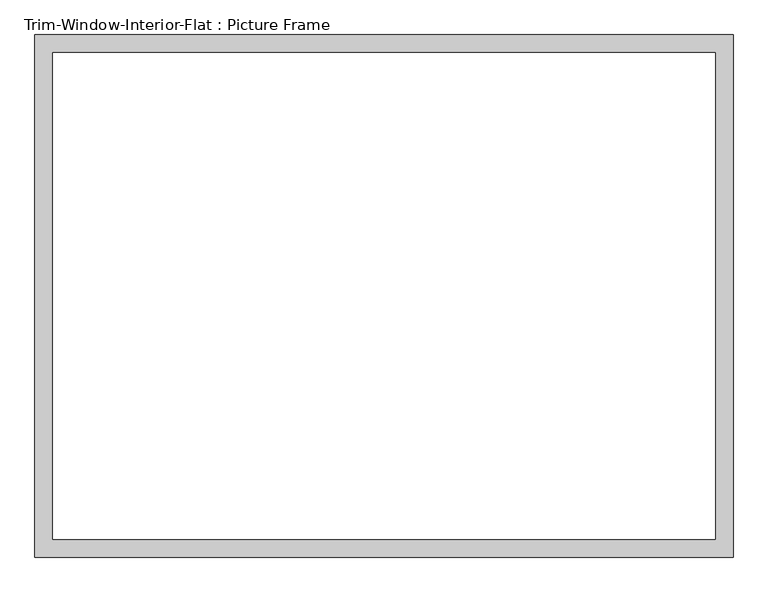
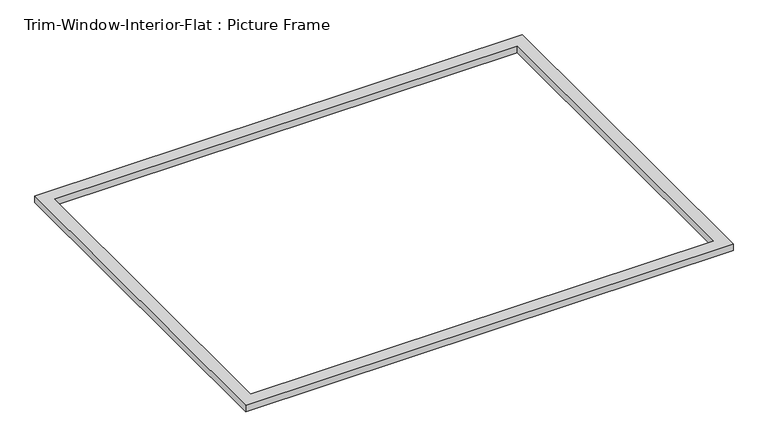
"""IFC4 building model written with IfcOpenShell, lengths in millimetres: proxy geometry, Trim-Window-Interior-Flat : Picture Frame."""

from ifc_helpers import new_model, si_unit, origin, origin_with_axes, place, context, project, spatial, polyline, outline, extrude, source, transform, mapped, element, save


def trim_window_interior_flat_picture_frame_e25f2530(model_context):
    return source(origin(), model_context, "Body", "SweptSolid", [
        extrude(outline(polyline([(1111.25, 44.45), (1111.25, -1619.25), (-1111.25, -1619.25), (-1111.25, 44.45), (1111.25, 44.45)]), holes=[polyline([(1054.1, -12.7), (-1054.1, -12.7), (-1054.1, -1562.1), (1054.1, -1562.1), (1054.1, -12.7)])]), origin_with_axes(), (0.0, 0.0, 1.0), 31.75),
    ])


if __name__ == "__main__":
    model = new_model("IFC4")
    model_context = context("Model", 3, world=origin())
    ifc_project = project(units=[si_unit("LENGTHUNIT", "METRE", prefix="MILLI")], contexts=[model_context])
    site = spatial("IfcSite", under=ifc_project)
    building = spatial("IfcBuilding", under=site)
    placement = place(None, origin())
    trim_window_interior_flat_picture_frame_shape = trim_window_interior_flat_picture_frame_e25f2530(model_context)
    element("IfcBuildingElementProxy", 1, Name="Trim-Window-Interior-Flat : Picture Frame", ObjectType="Trim-Window-Interior-Flat : Picture Frame", at=placement, inside=building, context=model_context, shape_type="MappedRepresentation", body=[
        mapped(trim_window_interior_flat_picture_frame_shape, transform((0.0, 0.0, 0.0), x_axis=(1.0, 0.0, 0.0), y_axis=(0.0, 1.0, 0.0), z_axis=(0.0, 0.0, 1.0))),
    ])
    save(model, "model.ifc")

# Revit data of these elements
# Type "Trim-Window-Interior-Flat : Picture Frame"
#   Trim Thickness_Picture Frame = 0' - 1 1/4"
#   Trim Width = 0' - 2 1/4"
#   Trim Thickness_with Sill = 0' - 0 3/4"
#   Sill Thickness = 0' - 1 1/4"
#   Opening Width [instance default] = 2' - 0"
#   Opening Height [instance default] = 3' - 0"
#   Default Elevation = 4' - 0"
#   Sill = no
#   Picture Frame = yes
#   Trim Material [instance default] = none
# Element 1 (IfcBuildingElementProxy, "Trim-Window-Interior-Flat : Picture Frame")
#   Opening Width = 7' - 0"
#   Opening Height = 5' - 2"
#   Trim Material = Wood - Stained
#   Materials on its faces: "Wood - Stained"
# Materials
#   "Wood - Stained": class "Wood", colour RGB 227 170 128, transparency 0, Cost = 0
